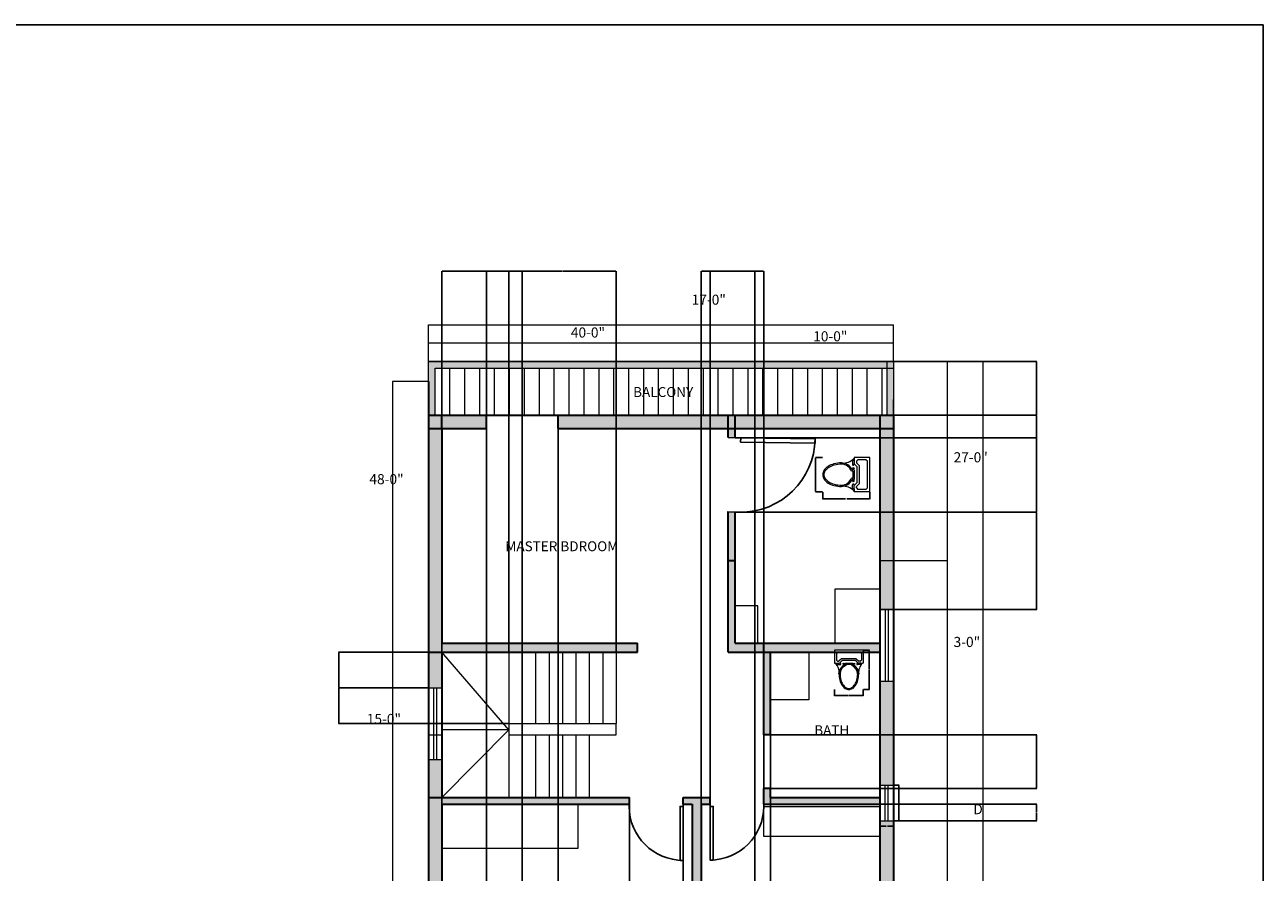
# Model space of a CAD drawing. Units: feet. Extents: x 2813 to 4435, y 1041 to 2557.
# Tile 6 of 6: x 3605 to 4435, y 1988 to 2557. Entities that reach past the tile are written whole.
import ezdxf

# ---------------------------------------------------------------- set-up
doc = ezdxf.new("R2010")
doc.units = ezdxf.units.FT
for name, color, linetype, lineweight in [('A-ANNO-DIMS', 2, 'Continuous', 18), ('A-ANNO-TTLB', 7, 'Continuous', 25), ('A-AREA-IDEN', 7, 'Continuous', 18), ('A-DOOR', 3, 'Continuous', 25), ('A-FLOR-CASE', 8, 'Continuous', 18), ('A-FLOR-FIXT', 9, 'Continuous', 18), ('A-FLOR-HRAL', 4, 'Continuous', 18), ('A-FLOR-STRS', 7, 'Continuous', 18), ('A-GLAZ', 4, 'Continuous', 18), ('A-WALL', 7, 'Continuous', 35), ('A-WALL-PATT', 252, 'Continuous', 13)]:
    doc.layers.add(name, color=color, linetype=linetype, lineweight=lineweight)
doc.styles.get("Standard").update_dxf_attribs({"font": 'arial.ttf'})
doc.dimstyles.get("Standard").update_dxf_attribs({"dimtxt": 0.18, "dimasz": 0.18, "dimexe": 0.18, "dimexo": 0.0625, "dimgap": 0.09, "dimtad": 0, "dimtih": 1, "dimtoh": 1, "dimdec": 4, "dimzin": 0, "dimdsep": 46, "dimtxsty": 'Standard', "dimcen": 0.09, "dimadec": 0, "dimazin": 0, "dimtfac": 1, "dimtdec": 4, "dimtofl": 0, "dimtmove": 0, "dimatfit": 3, "dimfxl": 1, "dimtolj": 1, "dimtzin": 0, "dimarcsym": 0})

# ---------------------------------------------------------------- blocks, each defined once
blk = doc.blocks.new('*U4')
for p, q in [((0, 0), (0, -5)), ((30, 0), (30, -5))]:
    blk.add_line(p, q)
blk.add_lwpolyline([(0, 0), (0, 30), (1.75, 30), (1.75, 0)], close=True)
blk.add_arc((0, 0), 30, 0, 90)
blk = doc.blocks.new('A$C098B081F')
for p, q in [((559, 762), (0, 762)), ((0, 762), (0, 508)), ((63, 724), (38, 698)), ((38, 698), (38, 571)), ((495, 724), (63, 724)), ((521, 698), (495, 724)), ((521, 698), (521, 571)), ((559, 762), (559, 508)), ((0, 508), (13, 508)), ((13, 508), (102, 508)), ((38, 571), (63, 546)), ((51, 508), (51, 483)), ((51, 508), (102, 508)), ((51, 483), (114, 483)), ((63, 546), (86, 546)), ((137, 597), (86, 546)), ((152, 559), (102, 508)), ((114, 508), (102, 508)), ((422, 597), (137, 597)), ((406, 559), (152, 559)), ((203, 508), (203, 479)), ((203, 508), (356, 508)), ((223, 488), (223, 466)), ((223, 488), (336, 488)), ((336, 488), (336, 466)), ((356, 508), (356, 479)), ((406, 559), (457, 508)), ((422, 597), (473, 546)), ((444, 508), (457, 508)), ((508, 483), (444, 483)), ((508, 508), (457, 508)), ((495, 546), (473, 546)), ((495, 546), (521, 571)), ((508, 508), (546, 508)), ((508, 508), (508, 483)), ((559, 508), (546, 508))]:
    blk.add_line(p, q)
for centre in [(178, 495), (381, 495)]:
    blk.add_circle(centre, 12.7)
for centre, radius, start, end in [((-137, 336), 228, 352.2011, 48.911), ((279, 305), 190, 113.5782, 180), ((279, 305), 170, 109.2456, 180), ((114, 495), 12.7, 270, 90), ((279, 305), 170, 0, 70.7544), ((279, 305), 190, 0, 66.4218), ((444, 495), 12.7, 90, 270), ((696, 336), 228, 131.089, 187.7989), ((575, 305), 486, 180, 194.5143), ((575, 305), 466, 180, 194.5143), ((-16, 305), 466, 345.4857, 360), ((-16, 305), 486, 345.4857, 360), ((429, 267), 335, 194.5143, 212.0054), ((429, 267), 315, 194.5143, 212.0054), ((337, 210), 227, 212.0054, 236.4659), ((337, 210), 207, 212.0054, 236.4659), ((279, 122), 122, 236.4659, 270), ((279, 122), 102, 236.4659, 270), ((279, 122), 102, 270, 303.5341), ((279, 122), 122, 270, 303.5341), ((222, 210), 207, 303.5341, 327.9946), ((222, 210), 227, 303.5341, 327.9946), ((130, 267), 315, 327.9946, 345.4857), ((130, 267), 335, 327.9946, 345.4857)]:
    blk.add_arc(centre, radius, start, end)
blk = doc.blocks.new('*U8')
blk.add_line((0, -15.75), (0, 15.75))
blk = doc.blocks.new('*U9')
at = {"layer": 'A-FLOR-HRAL', "color": 0, "linetype": 'ByBlock', "lineweight": -2, "transparency": 16777216}
for p in [(0, 0), (10, 0), (20, 0), (30, 0), (40, 0), (50, 0), (60, 0), (70, 0), (80, 0), (90, 0), (100, 0), (110, 0), (120, 0), (130, 0), (140, 0), (150, 0), (160, 0), (170, 0), (180, 0), (190, 0), (200, 0), (210, 0), (220, 0), (230, 0), (240, 0), (250, 0), (260, 0), (270, 0), (280, 0), (290, 0), (300, 0)]:
    blk.add_blockref('*U8', p, dxfattribs=at)
blk = doc.blocks.new('WINDOW-PLAN-WIDE')
for p, q in [((0, 0), (0, 9)), ((48, 0), (48, 9)), ((0, 5.5), (48, 5.5)), ((0, 3.5), (48, 3.5))]:
    blk.add_line(p, q)
blk = doc.blocks.new('WINDOW-PLAN-NARROW')
for p, q in [((0, 24), (9, 24)), ((3.5, 0), (3.5, 24)), ((5.5, 0), (5.5, 24)), ((0, 0), (9, 0))]:
    blk.add_line(p, q)
blk = doc.blocks.new('*D21')
at = {"layer": 'A-ANNO-DIMS', "color": 0, "lineweight": -2, "transparency": 16777216}
for p, q in [((4187.42, 2046.33), (4191.14, 2046.33)), ((4190.96, 2046.15), (4190.96, 2034.52)), ((4190.96, 2022.51), (4190.96, 2034.15)), ((4187.42, 2022.33), (4191.14, 2022.33))]:
    blk.add_line(p, q, dxfattribs=at)
at = {"layer": 'A-ANNO-DIMS', "color": 0, "transparency": 16777216}
for points in [[(4190.93, 2046.15), (4190.99, 2046.15), (4190.96, 2046.33)], [(4190.93, 2022.51), (4190.99, 2022.51), (4190.96, 2022.33)]]:
    blk.add_solid(points, dxfattribs=at)
at = {"layer": 'DEFPOINTS', "color": 0, "transparency": 16777216}
for p in [(4187.36, 2046.33), (4190.96, 2046.33), (4187.36, 2022.33)]:
    blk.add_point(p, dxfattribs=at)
at = {"layer": 'A-ANNO-DIMS', "color": 0, "transparency": 16777216, "insert": (4190.96, 2034.33), "char_height": 0.18, "attachment_point": 5}
blk.add_mtext('\\A1;NARROW WINDOW 24 TYP.', dxfattribs=at)
blk = doc.blocks.new('*D22')
at = {"layer": 'A-ANNO-DIMS', "color": 0, "lineweight": -2, "transparency": 16777216}
for p, q in [((4178.36, 2022.27), (4178.36, 2018.55)), ((4187.36, 2022.27), (4187.36, 2018.55)), ((4178.54, 2018.73), (4182.4, 2018.73)), ((4187.18, 2018.73), (4183.31, 2018.73))]:
    blk.add_line(p, q, dxfattribs=at)
at = {"layer": 'A-ANNO-DIMS', "color": 0, "transparency": 16777216}
for points in [[(4178.54, 2018.76), (4178.54, 2018.7), (4178.36, 2018.73)], [(4187.18, 2018.76), (4187.18, 2018.7), (4187.36, 2018.73)]]:
    blk.add_solid(points, dxfattribs=at)
at = {"layer": 'DEFPOINTS', "color": 0, "transparency": 16777216}
for p in [(4178.36, 2022.33), (4187.36, 2022.33), (4187.36, 2018.73)]:
    blk.add_point(p, dxfattribs=at)
at = {"layer": 'A-ANNO-DIMS', "color": 0, "transparency": 16777216, "insert": (4182.86, 2018.73), "char_height": 0.18, "attachment_point": 5}
blk.add_mtext('\\A1;9 TYP.', dxfattribs=at)
blk = doc.blocks.new('*D29')
at = {"layer": 'A-ANNO-DIMS', "color": 0, "lineweight": -2, "transparency": 16777216}
for p, q in [((4139.92, 2243.02), (4139.92, 2238.17)), ((4140.1, 2238.35), (4155.23, 2238.35)), ((4171.28, 2238.35), (4156.16, 2238.35)), ((4171.46, 2243.02), (4171.46, 2238.17))]:
    blk.add_line(p, q, dxfattribs=at)
at = {"layer": 'A-ANNO-DIMS', "color": 0, "transparency": 16777216}
for points in [[(4140.1, 2238.38), (4140.1, 2238.32), (4139.92, 2238.35)], [(4171.28, 2238.38), (4171.28, 2238.32), (4171.46, 2238.35)]]:
    blk.add_solid(points, dxfattribs=at)
at = {"layer": 'DEFPOINTS', "color": 0, "transparency": 16777216}
for p in [(4139.92, 2243.09), (4171.46, 2243.09), (4171.46, 2238.35)]:
    blk.add_point(p, dxfattribs=at)
at = {"layer": 'A-ANNO-DIMS', "color": 0, "transparency": 16777216, "insert": (4155.69, 2238.35), "char_height": 0.18, "attachment_point": 5}
blk.add_mtext('\\A1;WC 32', dxfattribs=at)
blk = doc.blocks.new('*D30')
at = {"layer": 'A-ANNO-DIMS', "color": 0, "lineweight": -2, "transparency": 16777216}
for p, q in [((4139.86, 2266.22), (4135.01, 2266.22)), ((4135.19, 2266.04), (4135.19, 2254.83)), ((4135.19, 2243.27), (4135.19, 2254.47)), ((4139.86, 2243.09), (4135.01, 2243.09))]:
    blk.add_line(p, q, dxfattribs=at)
at = {"layer": 'A-ANNO-DIMS', "color": 0, "transparency": 16777216}
for points in [[(4135.16, 2266.04), (4135.22, 2266.04), (4135.19, 2266.22)], [(4135.16, 2243.27), (4135.22, 2243.27), (4135.19, 2243.09)]]:
    blk.add_solid(points, dxfattribs=at)
at = {"layer": 'DEFPOINTS', "color": 0, "transparency": 16777216}
for p in [(4139.92, 2266.22), (4135.19, 2243.09), (4139.92, 2243.09)]:
    blk.add_point(p, dxfattribs=at)
at = {"layer": 'A-ANNO-DIMS', "color": 0, "transparency": 16777216, "insert": (4135.19, 2254.65), "char_height": 0.18, "attachment_point": 5}
blk.add_mtext('\\A1;23', dxfattribs=at)
blk = doc.blocks.new('*D31')
at = {"layer": 'A-ANNO-DIMS', "color": 0, "lineweight": -2, "transparency": 16777216}
for p, q in [((4167.23, 2136.91), (4171.31, 2136.91)), ((4171.13, 2136.73), (4171.13, 2123.86)), ((4171.13, 2110.63), (4171.13, 2123.5)), ((4167.23, 2110.45), (4171.31, 2110.45))]:
    blk.add_line(p, q, dxfattribs=at)
at = {"layer": 'A-ANNO-DIMS', "color": 0, "transparency": 16777216}
for points in [[(4171.1, 2136.73), (4171.16, 2136.73), (4171.13, 2136.91)], [(4171.1, 2110.63), (4171.16, 2110.63), (4171.13, 2110.45)]]:
    blk.add_solid(points, dxfattribs=at)
at = {"layer": 'DEFPOINTS', "color": 0, "transparency": 16777216}
for p in [(4167.17, 2136.91), (4171.13, 2136.91), (4167.17, 2110.45)]:
    blk.add_point(p, dxfattribs=at)
at = {"layer": 'A-ANNO-DIMS', "color": 0, "transparency": 16777216, "insert": (4171.13, 2123.68), "char_height": 0.18, "attachment_point": 5}
blk.add_mtext('\\A1;WC 26', dxfattribs=at)
blk = doc.blocks.new('*D32')
at = {"layer": 'A-ANNO-DIMS', "color": 0, "lineweight": -2, "transparency": 16777216}
for p, q in [((4147.77, 2110.39), (4147.77, 2106.3)), ((4147.95, 2106.48), (4157.26, 2106.48)), ((4166.99, 2106.48), (4157.68, 2106.48)), ((4167.17, 2110.39), (4167.17, 2106.3))]:
    blk.add_line(p, q, dxfattribs=at)
at = {"layer": 'A-ANNO-DIMS', "color": 0, "transparency": 16777216}
for points in [[(4147.95, 2106.51), (4147.95, 2106.45), (4147.77, 2106.48)], [(4166.99, 2106.51), (4166.99, 2106.45), (4167.17, 2106.48)]]:
    blk.add_solid(points, dxfattribs=at)
at = {"layer": 'DEFPOINTS', "color": 0, "transparency": 16777216}
for p in [(4147.77, 2110.45), (4167.17, 2110.45), (4167.17, 2106.48)]:
    blk.add_point(p, dxfattribs=at)
at = {"layer": 'A-ANNO-DIMS', "color": 0, "transparency": 16777216, "insert": (4157.47, 2106.48), "char_height": 0.18, "attachment_point": 5}
blk.add_mtext('\\A1;19', dxfattribs=at)
blk = doc.blocks.new('*D61')
at = {"layer": 'A-ANNO-DIMS', "color": 0, "lineweight": -2, "transparency": 16777216}
for p, q in [((3884.36, 2285.65), (3884.36, 2391.31)), ((3884.54, 2391.13), (3899.14, 2391.13)), ((3914.18, 2391.13), (3899.57, 2391.13)), ((3914.36, 2285.65), (3914.36, 2391.31))]:
    blk.add_line(p, q, dxfattribs=at)
at = {"layer": 'A-ANNO-DIMS', "color": 0, "transparency": 16777216}
for points in [[(3884.54, 2391.16), (3884.54, 2391.1), (3884.36, 2391.13)], [(3914.18, 2391.16), (3914.18, 2391.1), (3914.36, 2391.13)]]:
    blk.add_solid(points, dxfattribs=at)
at = {"layer": 'DEFPOINTS', "color": 0, "transparency": 16777216}
for p in [(3914.36, 2391.13), (3884.36, 2285.58), (3914.36, 2285.58)]:
    blk.add_point(p, dxfattribs=at)
at = {"layer": 'A-ANNO-DIMS', "color": 0, "transparency": 16777216, "insert": (3899.36, 2391.13), "char_height": 0.18, "attachment_point": 5}
blk.add_mtext('\\A1;30', dxfattribs=at)
blk = doc.blocks.new('*D62')
at = {"layer": 'A-ANNO-DIMS', "color": 0, "lineweight": -2, "transparency": 16777216}
for p, q in [((3914.36, 2285.52), (3914.36, 1691.4)), ((3962.36, 2285.52), (3962.36, 1691.4)), ((3914.54, 1691.58), (3938.13, 1691.58)), ((3962.18, 1691.58), (3938.58, 1691.58))]:
    blk.add_line(p, q, dxfattribs=at)
at = {"layer": 'A-ANNO-DIMS', "color": 0, "transparency": 16777216}
for points in [[(3914.54, 1691.61), (3914.54, 1691.55), (3914.36, 1691.58)], [(3962.18, 1691.61), (3962.18, 1691.55), (3962.36, 1691.58)]]:
    blk.add_solid(points, dxfattribs=at)
at = {"layer": 'DEFPOINTS', "color": 0, "transparency": 16777216}
for p in [(3914.36, 2285.58), (3962.36, 2285.58), (3962.36, 1691.58)]:
    blk.add_point(p, dxfattribs=at)
at = {"layer": 'A-ANNO-DIMS', "color": 0, "transparency": 16777216, "insert": (3938.36, 1691.58), "char_height": 0.18, "attachment_point": 5}
blk.add_mtext('\\A1;48', dxfattribs=at)
blk = doc.blocks.new('*D63')
at = {"layer": 'A-ANNO-DIMS', "color": 0, "lineweight": -2, "transparency": 16777216}
for p, q in [((4178.36, 2116.02), (4178.36, 1691.4)), ((4104.86, 2080.02), (4104.86, 1691.4)), ((4105.04, 1691.58), (4141.28, 1691.58)), ((4178.18, 1691.58), (4141.93, 1691.58))]:
    blk.add_line(p, q, dxfattribs=at)
at = {"layer": 'A-ANNO-DIMS', "color": 0, "transparency": 16777216}
for points in [[(4105.04, 1691.61), (4105.04, 1691.55), (4104.86, 1691.58)], [(4178.18, 1691.61), (4178.18, 1691.55), (4178.36, 1691.58)]]:
    blk.add_solid(points, dxfattribs=at)
at = {"layer": 'DEFPOINTS', "color": 0, "transparency": 16777216}
for p in [(4178.36, 2116.08), (4104.86, 2080.08), (4178.36, 1691.58)]:
    blk.add_point(p, dxfattribs=at)
at = {"layer": 'A-ANNO-DIMS', "color": 0, "transparency": 16777216, "insert": (4141.61, 1691.58), "char_height": 0.18, "attachment_point": 5}
blk.add_mtext('\\A1;73.5', dxfattribs=at)
blk = doc.blocks.new('*D64')
at = {"layer": 'A-ANNO-DIMS', "color": 0, "lineweight": -2, "transparency": 16777216}
for p, q in [((4178.42, 2294.58), (4283.54, 2294.58)), ((4283.36, 2294.4), (4283.36, 2229.51)), ((4283.36, 2164.26), (4283.36, 2229.15)), ((4178.42, 2164.08), (4283.54, 2164.08))]:
    blk.add_line(p, q, dxfattribs=at)
at = {"layer": 'A-ANNO-DIMS', "color": 0, "transparency": 16777216}
for points in [[(4283.33, 2294.4), (4283.39, 2294.4), (4283.36, 2294.58)], [(4283.33, 2164.26), (4283.39, 2164.26), (4283.36, 2164.08)]]:
    blk.add_solid(points, dxfattribs=at)
at = {"layer": 'DEFPOINTS', "color": 0, "transparency": 16777216}
for p in [(4178.36, 2294.58), (4178.36, 2164.08), (4283.36, 2164.08)]:
    blk.add_point(p, dxfattribs=at)
at = {"layer": 'A-ANNO-DIMS', "color": 0, "transparency": 16777216, "insert": (4283.36, 2229.33), "char_height": 0.18, "attachment_point": 5}
blk.add_mtext('\\A1;130.5', dxfattribs=at)
blk = doc.blocks.new('*D65')
at = {"layer": 'A-ANNO-DIMS', "color": 0, "lineweight": -2, "transparency": 16777216}
for p, q in [((3884.36, 1843.15), (3884.36, 2391.31)), ((3884.54, 2391.13), (3911.14, 2391.13)), ((3938.18, 2391.13), (3911.57, 2391.13)), ((3938.36, 1843.15), (3938.36, 2391.31))]:
    blk.add_line(p, q, dxfattribs=at)
at = {"layer": 'A-ANNO-DIMS', "color": 0, "transparency": 16777216}
for points in [[(3884.54, 2391.16), (3884.54, 2391.1), (3884.36, 2391.13)], [(3938.18, 2391.16), (3938.18, 2391.1), (3938.36, 2391.13)]]:
    blk.add_solid(points, dxfattribs=at)
at = {"layer": 'DEFPOINTS', "color": 0, "transparency": 16777216}
for p in [(3938.36, 2391.13), (3884.36, 1843.08), (3938.36, 1843.08)]:
    blk.add_point(p, dxfattribs=at)
at = {"layer": 'A-ANNO-DIMS', "color": 0, "transparency": 16777216, "insert": (3911.36, 2391.13), "char_height": 0.18, "attachment_point": 5}
blk.add_mtext('\\A1;54', dxfattribs=at)
blk = doc.blocks.new('*D66')
at = {"layer": 'A-ANNO-DIMS', "color": 0, "lineweight": -2, "transparency": 16777216}
for p, q in [((4058.36, 1843.15), (4058.36, 2391.31)), ((4058.54, 2391.13), (4076.14, 2391.13)), ((4094.18, 2391.13), (4076.57, 2391.13)), ((4094.36, 1843.15), (4094.36, 2391.31))]:
    blk.add_line(p, q, dxfattribs=at)
at = {"layer": 'A-ANNO-DIMS', "color": 0, "transparency": 16777216}
for points in [[(4058.54, 2391.16), (4058.54, 2391.1), (4058.36, 2391.13)], [(4094.18, 2391.16), (4094.18, 2391.1), (4094.36, 2391.13)]]:
    blk.add_solid(points, dxfattribs=at)
at = {"layer": 'DEFPOINTS', "color": 0, "transparency": 16777216}
for p in [(4094.36, 2391.13), (4058.36, 1843.08), (4094.36, 1843.08)]:
    blk.add_point(p, dxfattribs=at)
at = {"layer": 'A-ANNO-DIMS', "color": 0, "transparency": 16777216, "insert": (4076.36, 2391.13), "char_height": 0.18, "attachment_point": 5}
blk.add_mtext('\\A1;36', dxfattribs=at)
blk = doc.blocks.new('*D67')
at = {"layer": 'A-ANNO-DIMS', "color": 0, "lineweight": -2, "transparency": 16777216}
for p, q in [((3875.42, 2330.58), (4283.54, 2330.58)), ((4283.36, 2330.4), (4283.36, 2312.76)), ((4283.36, 2294.76), (4283.36, 2312.4)), ((3875.42, 2294.58), (4283.54, 2294.58))]:
    blk.add_line(p, q, dxfattribs=at)
at = {"layer": 'A-ANNO-DIMS', "color": 0, "transparency": 16777216}
for points in [[(4283.33, 2330.4), (4283.39, 2330.4), (4283.36, 2330.58)], [(4283.33, 2294.76), (4283.39, 2294.76), (4283.36, 2294.58)]]:
    blk.add_solid(points, dxfattribs=at)
at = {"layer": 'DEFPOINTS', "color": 0, "transparency": 16777216}
for p in [(3875.36, 2330.58), (3875.36, 2294.58), (4283.36, 2294.58)]:
    blk.add_point(p, dxfattribs=at)
at = {"layer": 'A-ANNO-DIMS', "color": 0, "transparency": 16777216, "insert": (4283.36, 2312.58), "char_height": 0.18, "attachment_point": 5}
blk.add_mtext('\\A1;36', dxfattribs=at)
blk = doc.blocks.new('*D68')
at = {"layer": 'A-ANNO-DIMS', "color": 0, "lineweight": -2, "transparency": 16777216}
for p, q in [((4010.36, 2033.52), (4010.36, 1691.4)), ((4046.36, 1995.76), (4046.36, 1691.4)), ((4010.54, 1691.58), (4028.14, 1691.58)), ((4046.18, 1691.58), (4028.57, 1691.58))]:
    blk.add_line(p, q, dxfattribs=at)
at = {"layer": 'A-ANNO-DIMS', "color": 0, "transparency": 16777216}
for points in [[(4010.54, 1691.61), (4010.54, 1691.55), (4010.36, 1691.58)], [(4046.18, 1691.61), (4046.18, 1691.55), (4046.36, 1691.58)]]:
    blk.add_solid(points, dxfattribs=at)
at = {"layer": 'DEFPOINTS', "color": 0, "transparency": 16777216}
for p in [(4010.36, 2033.58), (4046.36, 1995.82), (4046.36, 1691.58)]:
    blk.add_point(p, dxfattribs=at)
at = {"layer": 'A-ANNO-DIMS', "color": 0, "transparency": 16777216, "insert": (4028.36, 1691.58), "char_height": 0.18, "attachment_point": 5}
blk.add_mtext('\\A1;36', dxfattribs=at)
blk = doc.blocks.new('*D69')
at = {"layer": 'A-ANNO-DIMS', "color": 0, "lineweight": -2, "transparency": 16777216}
for p, q in [((4064.36, 2038.15), (4064.36, 2391.31)), ((4064.54, 2391.13), (4082.14, 2391.13)), ((4100.18, 2391.13), (4082.57, 2391.13)), ((4100.36, 2038.15), (4100.36, 2391.31))]:
    blk.add_line(p, q, dxfattribs=at)
at = {"layer": 'A-ANNO-DIMS', "color": 0, "transparency": 16777216}
for points in [[(4064.54, 2391.16), (4064.54, 2391.1), (4064.36, 2391.13)], [(4100.18, 2391.16), (4100.18, 2391.1), (4100.36, 2391.13)]]:
    blk.add_solid(points, dxfattribs=at)
at = {"layer": 'DEFPOINTS', "color": 0, "transparency": 16777216}
for p in [(4100.36, 2391.13), (4064.36, 2038.08), (4100.36, 2038.08)]:
    blk.add_point(p, dxfattribs=at)
at = {"layer": 'A-ANNO-DIMS', "color": 0, "transparency": 16777216, "insert": (4082.36, 2391.13), "char_height": 0.18, "attachment_point": 5}
blk.add_mtext('\\A1;36', dxfattribs=at)
blk = doc.blocks.new('*D70')
at = {"layer": 'A-ANNO-DIMS', "color": 0, "lineweight": -2, "transparency": 16777216}
for p, q in [((4104.92, 2080.08), (4283.54, 2080.08)), ((4283.36, 2079.9), (4283.36, 2062.26)), ((4283.36, 2044.26), (4283.36, 2061.9)), ((4104.92, 2044.08), (4283.54, 2044.08))]:
    blk.add_line(p, q, dxfattribs=at)
at = {"layer": 'A-ANNO-DIMS', "color": 0, "transparency": 16777216}
for points in [[(4283.33, 2079.9), (4283.39, 2079.9), (4283.36, 2080.08)], [(4283.33, 2044.26), (4283.39, 2044.26), (4283.36, 2044.08)]]:
    blk.add_solid(points, dxfattribs=at)
at = {"layer": 'DEFPOINTS', "color": 0, "transparency": 16777216}
for p in [(4104.86, 2080.08), (4104.86, 2044.08), (4283.36, 2044.08)]:
    blk.add_point(p, dxfattribs=at)
at = {"layer": 'A-ANNO-DIMS', "color": 0, "transparency": 16777216, "insert": (4283.36, 2062.08), "char_height": 0.18, "attachment_point": 5}
blk.add_mtext('\\A1;36', dxfattribs=at)
blk = doc.blocks.new('*D76')
at = {"layer": 'A-ANNO-DIMS', "color": 0, "lineweight": -2, "transparency": 16777216}
for p, q in [((3875.29, 2135.58), (3815.18, 2135.58)), ((3815.36, 2135.4), (3815.36, 2123.76)), ((3815.36, 2111.76), (3815.36, 2123.4)), ((3875.29, 2111.58), (3815.18, 2111.58))]:
    blk.add_line(p, q, dxfattribs=at)
at = {"layer": 'A-ANNO-DIMS', "color": 0, "transparency": 16777216}
for points in [[(3815.33, 2135.4), (3815.39, 2135.4), (3815.36, 2135.58)], [(3815.33, 2111.76), (3815.39, 2111.76), (3815.36, 2111.58)]]:
    blk.add_solid(points, dxfattribs=at)
at = {"layer": 'DEFPOINTS', "color": 0, "transparency": 16777216}
for p in [(3875.36, 2135.58), (3815.36, 2111.58), (3875.36, 2111.58)]:
    blk.add_point(p, dxfattribs=at)
at = {"layer": 'A-ANNO-DIMS', "color": 0, "transparency": 16777216, "insert": (3815.36, 2123.58), "char_height": 0.18, "attachment_point": 5}
blk.add_mtext('\\A1;24', dxfattribs=at)
blk = doc.blocks.new('*D77')
at = {"layer": 'A-ANNO-DIMS', "color": 0, "lineweight": -2, "transparency": 16777216}
for p, q in [((4178.42, 2033.58), (4283.54, 2033.58)), ((4283.36, 2033.4), (4283.36, 2028.14)), ((4283.36, 2022.51), (4283.36, 2027.78)), ((4187.42, 2022.33), (4283.54, 2022.33))]:
    blk.add_line(p, q, dxfattribs=at)
at = {"layer": 'A-ANNO-DIMS', "color": 0, "transparency": 16777216}
for points in [[(4283.33, 2033.4), (4283.39, 2033.4), (4283.36, 2033.58)], [(4283.33, 2022.51), (4283.39, 2022.51), (4283.36, 2022.33)]]:
    blk.add_solid(points, dxfattribs=at)
at = {"layer": 'DEFPOINTS', "color": 0, "transparency": 16777216}
for p in [(4178.36, 2033.58), (4283.36, 2033.58), (4187.36, 2022.33)]:
    blk.add_point(p, dxfattribs=at)
at = {"layer": 'A-ANNO-DIMS', "color": 0, "transparency": 16777216, "insert": (4283.36, 2027.96), "char_height": 0.18, "attachment_point": 5}
blk.add_mtext('\\A1;11.25', dxfattribs=at)
blk = doc.blocks.new('*D78')
at = {"layer": 'A-ANNO-DIMS', "color": 0, "lineweight": -2, "transparency": 16777216}
for p, q in [((3929.29, 2135.58), (3815.18, 2135.58)), ((3815.36, 2135.4), (3815.36, 2111.76)), ((3815.36, 2087.76), (3815.36, 2111.4)), ((3929.29, 2087.58), (3815.18, 2087.58))]:
    blk.add_line(p, q, dxfattribs=at)
at = {"layer": 'A-ANNO-DIMS', "color": 0, "transparency": 16777216}
for points in [[(3815.33, 2135.4), (3815.39, 2135.4), (3815.36, 2135.58)], [(3815.33, 2087.76), (3815.39, 2087.76), (3815.36, 2087.58)]]:
    blk.add_solid(points, dxfattribs=at)
at = {"layer": 'DEFPOINTS', "color": 0, "transparency": 16777216}
for p in [(3815.36, 2135.58), (3929.36, 2135.58), (3929.36, 2087.58)]:
    blk.add_point(p, dxfattribs=at)
at = {"layer": 'A-ANNO-DIMS', "color": 0, "transparency": 16777216, "insert": (3815.36, 2111.58), "char_height": 0.18, "attachment_point": 5}
blk.add_mtext('\\A1;48', dxfattribs=at)
blk = doc.blocks.new('*D79')
at = {"layer": 'A-ANNO-DIMS', "color": 0, "lineweight": -2, "transparency": 16777216}
for p, q in [((3929.36, 2135.65), (3929.36, 2391.31)), ((3929.54, 2391.13), (3965.14, 2391.13)), ((4001.18, 2391.13), (3965.57, 2391.13)), ((4001.36, 2135.65), (4001.36, 2391.31))]:
    blk.add_line(p, q, dxfattribs=at)
at = {"layer": 'A-ANNO-DIMS', "color": 0, "transparency": 16777216}
for points in [[(3929.54, 2391.16), (3929.54, 2391.1), (3929.36, 2391.13)], [(4001.18, 2391.16), (4001.18, 2391.1), (4001.36, 2391.13)]]:
    blk.add_solid(points, dxfattribs=at)
at = {"layer": 'DEFPOINTS', "color": 0, "transparency": 16777216}
for p in [(4001.36, 2391.13), (3929.36, 2135.58), (4001.36, 2135.58)]:
    blk.add_point(p, dxfattribs=at)
at = {"layer": 'A-ANNO-DIMS', "color": 0, "transparency": 16777216, "insert": (3965.36, 2391.13), "char_height": 0.18, "attachment_point": 5}
blk.add_mtext('\\A1;72', dxfattribs=at)
blk = doc.blocks.new('*D80')
at = {"layer": 'A-ANNO-DIMS', "color": 0, "lineweight": -2, "transparency": 16777216}
for p, q in [((4081.17, 2279.47), (4283.54, 2279.47)), ((4283.36, 2279.29), (4283.36, 2254.69)), ((4283.36, 2229.73), (4283.36, 2254.33)), ((4081.4, 2229.55), (4283.54, 2229.55))]:
    blk.add_line(p, q, dxfattribs=at)
at = {"layer": 'A-ANNO-DIMS', "color": 0, "transparency": 16777216}
for points in [[(4283.33, 2279.29), (4283.39, 2279.29), (4283.36, 2279.47)], [(4283.33, 2229.73), (4283.39, 2229.73), (4283.36, 2229.55)]]:
    blk.add_solid(points, dxfattribs=at)
at = {"layer": 'DEFPOINTS', "color": 0, "transparency": 16777216}
for p in [(4081.11, 2279.47), (4283.36, 2279.47), (4081.34, 2229.55)]:
    blk.add_point(p, dxfattribs=at)
at = {"layer": 'A-ANNO-DIMS', "color": 0, "transparency": 16777216, "insert": (4283.36, 2254.51), "char_height": 0.18, "attachment_point": 5}
blk.add_mtext('\\A1;49.92', dxfattribs=at)

msp = doc.modelspace()

# ---------------------------------------------------------------- hatches: boundary and pattern name
at = {"layer": 'A-WALL-PATT'}
h = msp.add_hatch(color=256, dxfattribs=at)
h.dxf.hatch_style = 1
h.paths.add_polyline_path([(4187.355, 2022.333), (4178.355, 2022.333), (4178.355, 2011.884), (4178.355, 1843.083), (4142.355, 1843.083), (4142.355, 1834.083), (4187.355, 1834.083)])
h.paths.add_polyline_path([(4187.355, 2116.083), (4178.355, 2116.083), (4178.355, 2046.333), (4187.355, 2046.333)])
h.paths.add_polyline_path([(4178.355, 2038.083), (4104.855, 2038.083), (4104.855, 2044.083), (4100.355, 2044.083), (4100.355, 2038.083), (4100.355, 2033.583), (4178.355, 2033.583)])
h.paths.add_polyline_path([(4064.355, 2038.083), (4046.355, 2038.083), (4046.355, 2033.583), (4052.355, 2033.583), (4052.355, 1763.583), (4058.355, 1763.583), (4058.355, 2033.583), (4064.355, 2033.583)])
h.paths.add_polyline_path([(4010.355, 2038.083), (3875.355, 2038.083), (3875.355, 1837.083), (3884.355, 1837.083), (3884.355, 2033.583), (3975.707, 2033.583), (4010.355, 2033.583)])
h.paths.add_polyline_path([(3884.355, 2063.583), (3875.355, 2063.583), (3875.355, 2038.083), (3884.355, 2038.083)])
h.paths.add_polyline_path([(3884.355, 2135.583), (3875.355, 2135.583), (3875.355, 2111.583), (3884.355, 2111.583)])
h.paths.add_polyline_path([(4015.739, 2141.583), (3884.355, 2141.583), (3884.355, 2285.583), (3875.355, 2285.583), (3875.355, 2135.583), (3884.355, 2135.583), (4015.739, 2135.583)])
h.paths.add_polyline_path([(4187.355, 2285.583), (4178.355, 2285.583), (4178.355, 2197.083), (4187.355, 2197.083)])
h.paths.add_polyline_path([(4187.355, 2197.083), (4178.355, 2197.083), (4178.355, 2164.083), (4187.355, 2164.083)])
h.paths.add_polyline_path([(4178.355, 2141.583), (4148.404, 2141.583), (4100.355, 2141.583), (4100.355, 2135.583), (4147.767, 2135.583), (4147.767, 2136.905), (4167.166, 2136.905), (4167.166, 2135.583), (4178.355, 2135.583)])
h.paths.add_polyline_path([(4100.355, 2141.583), (4081.108, 2141.583), (4081.108, 2166.684), (4081.108, 2197.083), (4076.608, 2197.083), (4076.608, 2135.583), (4100.355, 2135.583)])
h.paths.add_polyline_path([(4081.108, 2229.555), (4076.608, 2229.616), (4076.608, 2197.083), (4081.108, 2197.083)])
h.paths.add_polyline_path([(4081.108, 2294.583), (4076.608, 2294.583), (4076.608, 2285.583), (4081.108, 2285.583)])
h.paths.add_polyline_path([(4081.108, 2285.583), (4076.608, 2285.583), (4076.608, 2279.532), (4081.108, 2279.471)])
h.paths.add_polyline_path([(4076.608, 2294.583), (3962.355, 2294.583), (3962.355, 2285.583), (4076.608, 2285.583)])
h.paths.add_polyline_path([(4178.355, 2294.583), (4081.108, 2294.583), (4081.108, 2285.583), (4178.355, 2285.583)])
h.paths.add_polyline_path([(4187.355, 2294.583), (4178.355, 2294.583), (4178.355, 2285.583), (4187.355, 2285.583)])
h.paths.add_polyline_path([(3914.355, 2294.583), (3884.355, 2294.583), (3884.355, 2285.583), (3914.355, 2285.583)])
h.paths.add_polyline_path([(3884.355, 2294.583), (3875.355, 2294.583), (3875.355, 2285.583), (3884.355, 2285.583)])
h.paths.add_polyline_path([(4182.855, 2330.583), (3875.355, 2330.583), (3875.355, 2294.583), (3879.855, 2294.583), (3879.855, 2326.083), (4182.855, 2326.083)])
h.paths.add_polyline_path([(4187.355, 2330.583), (4182.855, 2330.583), (4182.855, 2326.083), (4187.355, 2326.083)])
h.paths.add_polyline_path([(4187.355, 2326.083), (4182.855, 2326.083), (4182.855, 2294.583), (4187.355, 2294.583)])
h.paths.add_polyline_path([(4052.355, 1843.083), (4046.355, 1843.083), (3986.355, 1843.083), (3986.355, 1837.083), (4046.355, 1837.083), (4052.355, 1837.083)])
h.paths.add_polyline_path([(4094.355, 1843.083), (4058.355, 1843.083), (4058.355, 1834.083), (4094.355, 1834.083)])
h.paths.add_polyline_path([(3938.355, 1843.083), (3884.355, 1843.083), (3884.355, 1837.083), (3938.355, 1837.083)], flags=17)
h = msp.add_hatch(color=256, dxfattribs=at)
h.dxf.hatch_style = 1
h.paths.add_polyline_path([(4104.855, 2135.583), (4100.355, 2135.583), (4100.355, 2080.083), (4104.855, 2080.083)])

# ---------------------------------------------------------------- linework, layer by layer
at = {"layer": 'A-ANNO-DIMS'}
for p, q in [((3875.355, 2355.125), (4187.355, 2355.125)), ((3875.355, 2330.583), (3875.355, 2355.125)), ((4187.355, 2330.583), (4187.355, 2355.125)), ((3875.355, 2343.125), (4187.355, 2343.125)), ((4187.355, 2330.583), (4247.355, 2330.583)), ((4223.355, 2330.583), (4223.355, 2197.083)), ((4247.355, 2330.583), (4247.355, 1834.083)), ((3875.355, 2317.195), (3851.355, 2317.195)), ((3851.355, 2317.195), (3851.355, 1763.583)), ((4223.355, 2317.195), (4223.355, 1834.083)), ((3875.355, 2111.583), (3875.355, 2294.583)), ((4178.355, 2197.083), (4223.355, 2197.083))]:
    msp.add_line(p, q, dxfattribs=at)
at = {"layer": 'A-ANNO-TTLB'}
for p, q in [((2933.466, 2556.562), (4435.474, 2556.562)), ((4435.474, 2556.562), (4435.474, 1041.465))]:
    msp.add_line(p, q, dxfattribs=at)
at = {"layer": 'A-FLOR-CASE'}
for points in [[(3884.355, 2033.583), (3975.707, 2033.583), (3975.707, 2003.88), (3884.355, 2003.88)], [(4100.383, 2032.078), (4178.355, 2032.078), (4178.355, 2011.884), (4100.383, 2011.884)]]:
    msp.add_lwpolyline(points, close=True, dxfattribs=at)
at = {"layer": 'A-FLOR-FIXT'}
for points in [[(4178.355, 2141.583), (4148.404, 2141.583), (4148.404, 2177.987), (4178.355, 2177.987)], [(4104.855, 2135.583), (4130.593, 2135.583), (4130.593, 2103.519), (4104.855, 2103.519)]]:
    msp.add_lwpolyline(points, close=True, dxfattribs=at)
msp.add_lwpolyline([(4096.494, 2141.583), (4096.494, 2166.684), (4081.108, 2166.684), (4081.108, 2141.583)], dxfattribs=at)
at = {"layer": 'A-FLOR-HRAL'}
for p, q in [((3875.355, 2294.583), (3875.355, 2330.583)), ((3875.355, 2330.583), (4187.355, 2330.583)), ((4182.855, 2330.583), (4182.855, 2294.583)), ((4187.355, 2330.583), (4187.355, 2294.583)), ((3879.855, 2326.083), (4187.355, 2326.083)), ((4187.355, 2294.583), (4187.355, 2305.195))]:
    msp.add_line(p, q, dxfattribs=at)
at = {"layer": 'A-FLOR-STRS'}
for p, q in [((3929.355, 2083.521), (3884.355, 2135.583)), ((3929.355, 2135.583), (3929.355, 2038.083)), ((3938.355, 2135.583), (3938.355, 2087.583)), ((3947.355, 2135.583), (3947.355, 2087.583)), ((3956.355, 2135.583), (3956.355, 2087.583)), ((3965.355, 2135.583), (3965.355, 2087.583)), ((3974.355, 2135.583), (3974.355, 2087.583)), ((3983.355, 2135.583), (3983.355, 2087.583)), ((3992.355, 2135.583), (3992.355, 2087.583)), ((4001.355, 2135.583), (4001.355, 2087.583)), ((3929.355, 2087.583), (4001.355, 2087.583)), ((4001.355, 2080.083), (4001.355, 2087.583)), ((3875.355, 2080.083), (3884.355, 2080.083)), ((3929.355, 2083.521), (3884.355, 2083.521)), ((3929.355, 2083.521), (3884.355, 2038.083)), ((3929.355, 2080.083), (3983.355, 2080.083)), ((3938.355, 2080.083), (3938.355, 2038.083)), ((3947.355, 2080.083), (3947.355, 2038.083)), ((3956.355, 2080.083), (3956.355, 2038.083)), ((3965.355, 2080.083), (3965.355, 2038.083)), ((3974.355, 2080.083), (3974.355, 2038.083)), ((3983.355, 2080.083), (3983.355, 2038.083)), ((3983.355, 2080.083), (4001.355, 2080.083))]:
    msp.add_line(p, q, dxfattribs=at)
at = {"layer": 'A-WALL'}
for p, q in [((3875.355, 2317.195), (3875.355, 1763.583)), ((3875.355, 2294.583), (4187.355, 2294.583)), ((3884.355, 2285.583), (3884.355, 2294.583)), ((3914.355, 2285.583), (3914.355, 2294.583)), ((3962.355, 2285.583), (3962.355, 2294.583)), ((4076.608, 2279.532), (4076.608, 2294.583)), ((4081.108, 2279.471), (4081.108, 2294.583)), ((4178.355, 2294.583), (4178.355, 1843.083)), ((4187.355, 2294.583), (4187.355, 1834.083)), ((3875.355, 2285.583), (3914.355, 2285.583)), ((3884.355, 2285.583), (3884.355, 2141.583)), ((3962.355, 2285.583), (4187.355, 2285.583)), ((4076.608, 2135.583), (4076.608, 2229.616)), ((4081.108, 2141.583), (4081.108, 2229.555)), ((4076.608, 2197.083), (4081.108, 2197.083)), ((3875.355, 2135.583), (4015.739, 2135.583)), ((3884.355, 2141.583), (4015.739, 2141.583)), ((3884.355, 2135.583), (3884.355, 2038.083)), ((4015.739, 2135.583), (4015.739, 2141.583)), ((4076.608, 2135.583), (4178.355, 2135.583)), ((4081.108, 2141.583), (4178.355, 2141.583)), ((4100.355, 2080.083), (4100.355, 2141.583)), ((4104.855, 2080.083), (4104.855, 2135.583)), ((4104.855, 2080.083), (4100.355, 2080.083)), ((4100.355, 2038.083), (4100.355, 2044.083)), ((4104.855, 2044.083), (4100.355, 2044.083)), ((4104.855, 2038.083), (4104.855, 2044.083)), ((3875.355, 2038.083), (4010.355, 2038.083)), ((4010.355, 2033.583), (4010.355, 2038.083)), ((4046.355, 2033.583), (4046.355, 2038.083)), ((4046.355, 2038.083), (4064.355, 2038.083)), ((4064.355, 2033.583), (4064.355, 2038.083)), ((4100.355, 2033.583), (4100.355, 2038.083)), ((4104.855, 2038.083), (4178.355, 2038.083)), ((3884.355, 2033.583), (3920.355, 2033.583)), ((3884.355, 2033.583), (3884.355, 1763.583)), ((3920.355, 2033.583), (4010.355, 2033.583)), ((4046.355, 2033.583), (4052.355, 2033.583)), ((4052.355, 2033.583), (4052.355, 1763.583)), ((4058.355, 2033.583), (4058.355, 1739.583)), ((4058.355, 2033.583), (4064.355, 2033.583)), ((4100.355, 2033.583), (4178.355, 2033.583))]:
    msp.add_line(p, q, dxfattribs=at)

# ---------------------------------------------------------------- block references
at = {"layer": 'A-DOOR'}
for p, xscale, yscale, zscale, rotation in [((4084.926, 2279.419), 1.6637245636514, 1.6637245636514, 1.6637245636514, 269.2201969845799), ((4046.355, 2032.046), 1.207415516413446, 1.207415516413446, 1.207415516413446, 180), ((4064.355, 2032.078), -1.200919304997554, 1.200919304997554, 1.200919304997554, 180)]:
    msp.add_blockref('*U4', p, dxfattribs=dict(at, xscale=xscale, yscale=yscale, zscale=zscale, rotation=rotation))
at = {"layer": 'A-FLOR-FIXT', "xscale": 0.0413985319535216, "yscale": 0.0413985319535216, "zscale": 0.0413985319535216, "rotation": 270}
msp.add_blockref('A$C098B081F', (4139.918, 2266.219), dxfattribs=at)
at = {"layer": 'A-FLOR-FIXT', "xscale": 0.0347146650528752, "yscale": 0.0347146650528752, "zscale": 0.0347146650528752}
msp.add_blockref('A$C098B081F', (4147.767, 2110.453), dxfattribs=at)
at = {"layer": 'A-FLOR-HRAL'}
msp.add_blockref('*U9', (3879.855, 2310.333), dxfattribs=at)
at = {"layer": 'A-GLAZ'}
for p, rotation in [((4178.356, 2164.083), 269.9999999999975), ((3875.356, 2111.583), 269.9999999999986)]:
    msp.add_blockref('WINDOW-PLAN-WIDE', p, dxfattribs=dict(at, rotation=rotation))
msp.add_blockref('WINDOW-PLAN-NARROW', (4178.355, 2022.333), dxfattribs=at)

# ---------------------------------------------------------------- texts
at = {"layer": 'A-ANNO-DIMS', "char_height": 6.7726, "attachment_point": 1}
for s, insert in [('17-0" ', (4052.007, 2375.469)), ('40-0" ', (3970.945, 2353.449)), ('10-0" ', (4133.535, 2350.881)), ('27-0" ', (4227.726, 2269.694)), ('48-0" ', (3835.801, 2255.039)), ('3-0" ', (4227.726, 2145.786)), ('15-0"', (3834.05, 2094.081)), ('D ', (4240.956, 2033.565))]:
    msp.add_mtext_dynamic_manual_height_columns(s, width=22.46964, gutter_width=33.863, heights=[0], dxfattribs=dict(at, insert=insert))
at = {"layer": 'A-AREA-IDEN', "attachment_point": 1}
for s, insert, char_height in [('BALCONY', (4012.764, 2313.443), 6.652), ('MASTER BDROOM', (3927.07, 2209.937), 6.65198), ('BATH', (4134.257, 2086.527), 6.652)]:
    msp.add_mtext_dynamic_manual_height_columns(s, width=109.65837, gutter_width=33.26, heights=[0], dxfattribs=dict(at, insert=insert, char_height=char_height))

# ---------------------------------------------------------------- dimensions: what is measured, and where the dimension line sits
at = {"layer": 'A-ANNO-DIMS'}
for base, p1, p2, override, picture, middle in [((3914.355, 2391.125), (3884.355, 2285.583), (3914.355, 2285.583), {"dimdec": 0, "dimlfac": 1, "dimrnd": 0, "dimzin": 0, "dimdsep": 46, "dimlunit": 2}, '*D61', (3899.355, 2391.125)), ((3938.355, 2391.125), (3884.355, 1843.083), (3938.355, 1843.083), {"dimdec": 0, "dimlfac": 1, "dimrnd": 0, "dimzin": 0, "dimdsep": 46, "dimlunit": 2}, '*D65', (3911.355, 2391.125)), ((4001.355, 2391.125), (3929.355, 2135.583), (4001.355, 2135.583), {"dimdec": 0, "dimlfac": 1, "dimrnd": 0, "dimzin": 0, "dimdsep": 46, "dimlunit": 2}, '*D79', (3965.355, 2391.125)), ((4094.355, 2391.125), (4058.355, 1843.083), (4094.355, 1843.083), {"dimdec": 0, "dimlfac": 1, "dimrnd": 0, "dimzin": 0, "dimdsep": 46, "dimlunit": 2}, '*D66', (4076.355, 2391.125)), ((4100.355, 2391.125), (4064.355, 2038.083), (4100.355, 2038.083), {"dimdec": 0, "dimlfac": 1, "dimrnd": 0, "dimzin": 0, "dimdsep": 46, "dimlunit": 2}, '*D69', (4082.355, 2391.125)), ((3962.355, 1691.583), (3914.355, 2285.583), (3962.355, 2285.583), {"dimdec": 0, "dimlfac": 1, "dimrnd": 0, "dimzin": 0, "dimdsep": 46, "dimlunit": 2}, '*D62', (3938.355, 1691.583)), ((4178.355, 1691.583), (4104.855, 2080.083), (4178.355, 2116.083), {"dimdec": 1, "dimlfac": 1, "dimrnd": 0, "dimzin": 0, "dimdsep": 46, "dimlunit": 2}, '*D63', (4141.605, 1691.583)), ((4167.166, 2106.485), (4147.767, 2110.453), (4167.166, 2110.453), {"dimdec": 0, "dimlfac": 1, "dimrnd": 0, "dimzin": 0, "dimdsep": 46, "dimlunit": 2}, '*D32', (4157.466, 2106.485)), ((4046.355, 1691.583), (4010.355, 2033.583), (4046.355, 1995.823), {"dimdec": 0, "dimlfac": 1, "dimrnd": 0, "dimzin": 0, "dimdsep": 46, "dimlunit": 2}, '*D68', (4028.355, 1691.583))]:
    dim = msp.add_linear_dim(base=base, p1=p1, p2=p2, dimstyle='Standard', override=override, dxfattribs=at)
    dim.commit()
    dim.dimension.update_dxf_attribs({"geometry": picture, "text_midpoint": middle})
for base, p1, p2, angle, override, picture, middle in [((4283.355, 2294.583), (3875.355, 2330.583), (3875.355, 2294.583), 90, {"dimdec": 0, "dimlfac": 1, "dimrnd": 0, "dimzin": 0, "dimdsep": 46, "dimlunit": 2}, '*D67', (4283.355, 2312.583)), ((4283.355, 2164.083), (4178.355, 2294.583), (4178.355, 2164.083), 90, {"dimdec": 1, "dimlfac": 1, "dimrnd": 0, "dimzin": 0, "dimdsep": 46, "dimlunit": 2}, '*D64', (4283.355, 2229.333)), ((4283.355, 2279.471), (4081.335, 2229.552), (4081.108, 2279.471), 90, {"dimdec": 2, "dimlfac": 1, "dimrnd": 0, "dimzin": 0, "dimdsep": 46, "dimlunit": 2}, '*D80', (4283.355, 2254.511)), ((4135.187, 2243.085), (4139.918, 2266.219), (4139.918, 2243.085), 270, {"dimdec": 0, "dimlfac": 1, "dimrnd": 0, "dimzin": 0, "dimdsep": 46, "dimlunit": 2}, '*D30', (4135.187, 2254.652)), ((3815.355, 2111.583), (3875.355, 2135.583), (3875.355, 2111.583), 90, {"dimdec": 0, "dimlfac": 1, "dimrnd": 0, "dimzin": 0, "dimdsep": 46, "dimlunit": 2}, '*D76', (3815.355, 2123.583)), ((3815.355, 2135.583), (3929.355, 2087.583), (3929.355, 2135.583), 90, {"dimdec": 0, "dimlfac": 1, "dimrnd": 0, "dimzin": 0, "dimdsep": 46, "dimlunit": 2}, '*D78', (3815.355, 2111.583)), ((4283.355, 2044.083), (4104.855, 2080.083), (4104.855, 2044.083), 90, {"dimdec": 0, "dimlfac": 1, "dimrnd": 0, "dimzin": 0, "dimdsep": 46, "dimlunit": 2}, '*D70', (4283.355, 2062.083)), ((4283.355, 2033.583), (4187.355, 2022.333), (4178.355, 2033.583), 90, {"dimdec": 2, "dimlfac": 1, "dimrnd": 0, "dimzin": 0, "dimdsep": 46, "dimlunit": 2}, '*D77', (4283.355, 2027.958))]:
    dim = msp.add_linear_dim(base=base, p1=p1, p2=p2, angle=angle, dimstyle='Standard', override=override, dxfattribs=at)
    dim.commit()
    dim.dimension.update_dxf_attribs({"geometry": picture, "text_midpoint": middle})
for base, p1, p2, text, picture, middle in [((4171.464, 2238.353), (4139.918, 2243.085), (4171.464, 2243.085), 'WC <>', '*D29', (4155.691, 2238.353)), ((4187.355, 2018.733), (4178.355, 2022.333), (4187.355, 2022.333), '<> TYP.', '*D22', (4182.855, 2018.733))]:
    dim = msp.add_linear_dim(base=base, p1=p1, p2=p2, text=text, dimstyle='Standard', override={"dimdec": 0, "dimlfac": 1, "dimrnd": 0, "dimzin": 0, "dimdsep": 46, "dimlunit": 2}, dxfattribs=at)
    dim.commit()
    dim.dimension.update_dxf_attribs({"geometry": picture, "text_midpoint": middle})
for base, p1, p2, text, picture, middle in [((4171.134, 2136.905), (4167.166, 2110.453), (4167.166, 2136.905), 'WC <>', '*D31', (4171.134, 2123.679)), ((4190.955, 2046.333), (4187.355, 2022.333), (4187.355, 2046.333), 'NARROW WINDOW <> TYP.', '*D21', (4190.955, 2034.333))]:
    dim = msp.add_linear_dim(base=base, p1=p1, p2=p2, angle=90, text=text, dimstyle='Standard', override={"dimdec": 0, "dimlfac": 1, "dimrnd": 0, "dimzin": 0, "dimdsep": 46, "dimlunit": 2}, dxfattribs=at)
    dim.commit()
    dim.dimension.update_dxf_attribs({"geometry": picture, "text_midpoint": middle})

doc.saveas('drawing.dxf')
